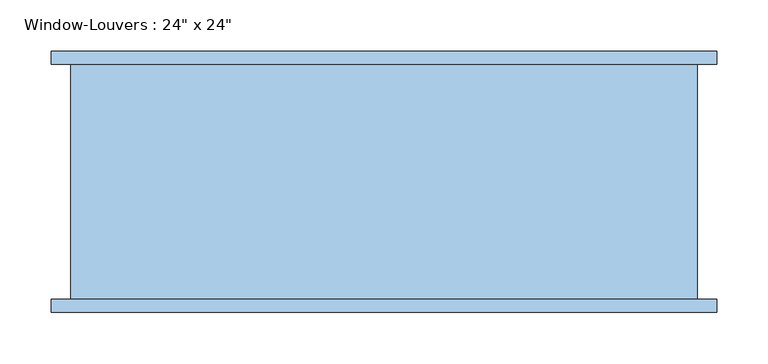
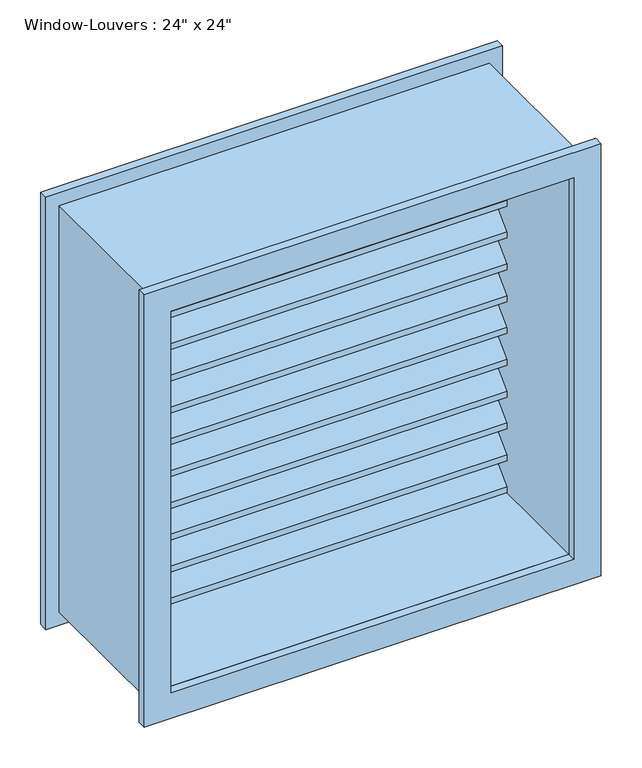
"""IFC4 building model written with IfcOpenShell, lengths in millimetres: window geometry."""

from ifc_helpers import new_model, si_unit, frame, origin, place, context, project, spatial, polyline, outline, extrude, source, transform, mapped, element, save


def window_f2d8fef0(model_context):
    return source(origin(), model_context, "Body", "SweptSolid", [
        extrude(outline(polyline([(107.95, 1419.1754778), (107.95, 1410.1952217), (69.85, 1448.2952217), (31.75, 1410.1952217), (31.75, 1419.1754778), (69.85, 1457.2754778), (107.95, 1419.1754778)])), frame((-285.75, 0.0, 0.0), z_axis=(1.0, 0.0, 0.0), x_axis=(0.0, 1.0, 0.0)), (0.0, 0.0, 1.0), 571.5),
        extrude(outline(polyline([(107.95, 1371.5009557), (107.95, 1362.5206995), (69.85, 1400.6206995), (31.75, 1362.5206995), (31.75, 1371.5009557), (69.85, 1409.6009557), (107.95, 1371.5009557)])), frame((-285.75, 0.0, 0.0), z_axis=(1.0, 0.0, 0.0), x_axis=(0.0, 1.0, 0.0)), (0.0, 0.0, 1.0), 571.5),
        extrude(outline(polyline([(107.95, 1323.8264335), (107.95, 1314.8461774), (69.85, 1352.9461774), (31.75, 1314.8461774), (31.75, 1323.8264335), (69.85, 1361.9264335), (107.95, 1323.8264335)])), frame((-285.75, 0.0, 0.0), z_axis=(1.0, 0.0, 0.0), x_axis=(0.0, 1.0, 0.0)), (0.0, 0.0, 1.0), 571.5),
        extrude(outline(polyline([(107.95, 1276.1519113), (107.95, 1267.1716552), (69.85, 1305.2716552), (31.75, 1267.1716552), (31.75, 1276.1519113), (69.85, 1314.2519113), (107.95, 1276.1519113)])), frame((-285.75, 0.0, 0.0), z_axis=(1.0, 0.0, 0.0), x_axis=(0.0, 1.0, 0.0)), (0.0, 0.0, 1.0), 571.5),
        extrude(outline(polyline([(107.95, 1228.4773891), (107.95, 1219.497133), (69.85, 1257.597133), (31.75, 1219.497133), (31.75, 1228.4773891), (69.85, 1266.5773891), (107.95, 1228.4773891)])), frame((-285.75, 0.0, 0.0), z_axis=(1.0, 0.0, 0.0), x_axis=(0.0, 1.0, 0.0)), (0.0, 0.0, 1.0), 571.5),
        extrude(outline(polyline([(107.95, 1180.802867), (107.95, 1171.8226109), (69.85, 1209.9226109), (31.75, 1171.8226109), (31.75, 1180.802867), (69.85, 1218.902867), (107.95, 1180.802867)])), frame((-285.75, 0.0, 0.0), z_axis=(1.0, 0.0, 0.0), x_axis=(0.0, 1.0, 0.0)), (0.0, 0.0, 1.0), 571.5),
        extrude(outline(polyline([(107.95, 1133.1283448), (107.95, 1124.1480887), (69.85, 1162.2480887), (31.75, 1124.1480887), (31.75, 1133.1283448), (69.85, 1171.2283448), (107.95, 1133.1283448)])), frame((-285.75, 0.0, 0.0), z_axis=(1.0, 0.0, 0.0), x_axis=(0.0, 1.0, 0.0)), (0.0, 0.0, 1.0), 571.5),
        extrude(outline(polyline([(107.95, 1085.4538226), (107.95, 1076.4735665), (69.85, 1114.5735665), (31.75, 1076.4735665), (31.75, 1085.4538226), (69.85, 1123.5538226), (107.95, 1085.4538226)])), frame((-285.75, 0.0, 0.0), z_axis=(1.0, 0.0, 0.0), x_axis=(0.0, 1.0, 0.0)), (0.0, 0.0, 1.0), 571.5),
        extrude(outline(polyline([(107.95, 1037.7793005), (107.95, 1028.7990443), (69.85, 1066.8990443), (31.75, 1028.7990443), (31.75, 1037.7793005), (69.85, 1075.8793005), (107.95, 1037.7793005)])), frame((-285.75, 0.0, 0.0), z_axis=(1.0, 0.0, 0.0), x_axis=(0.0, 1.0, 0.0)), (0.0, 0.0, 1.0), 571.5),
        extrude(outline(polyline([(107.95, 990.1047783), (107.95, 981.1245222), (69.85, 1019.2245222), (31.75, 981.1245222), (31.75, 990.1047783), (69.85, 1028.2047783), (107.95, 990.1047783)])), frame((-285.75, 0.0, 0.0), z_axis=(1.0, 0.0, 0.0), x_axis=(0.0, 1.0, 0.0)), (0.0, 0.0, 1.0), 571.5),
        extrude(outline(polyline([(107.95, 1466.85), (107.95, 1457.8697439), (69.85, 1495.9697439), (31.75, 1457.8697439), (31.75, 1466.85), (69.85, 1504.95), (107.95, 1466.85)])), frame((-285.75, 0.0, 0.0), z_axis=(1.0, 0.0, 0.0), x_axis=(0.0, 1.0, 0.0)), (0.0, 0.0, 1.0), 571.5),
        extrude(outline(polyline([(107.95, 942.4302561), (107.95, 933.45), (69.85, 971.55), (31.75, 933.45), (31.75, 942.4302561), (69.85, 980.5302561), (107.95, 942.4302561)])), frame((-285.75, 0.0, 0.0), z_axis=(1.0, 0.0, 0.0), x_axis=(0.0, 1.0, 0.0)), (0.0, 0.0, 1.0), 571.5),
        extrude(outline(polyline([(1524.0, 304.8), (1524.0, -304.8), (914.4, -304.8), (914.4, 304.8), (1524.0, 304.8)]), holes=[polyline([(1504.95, 285.75), (933.45, 285.75), (933.45, -285.75), (1504.95, -285.75), (1504.95, 285.75)])]), frame((0.0, -120.65, 0.0), z_axis=(0.0, 1.0, 0.0), x_axis=(0.0, 0.0, 1.0)), (0.0, 0.0, 1.0), 228.6),
        extrude(outline(polyline([(1543.05, 323.85), (1543.05, -323.85), (895.35, -323.85), (895.35, 323.85), (1543.05, 323.85)]), holes=[polyline([(1504.95, 285.75), (933.45, 285.75), (933.45, -285.75), (1504.95, -285.75), (1504.95, 285.75)])]), frame((0.0, -133.35, 0.0), z_axis=(0.0, 1.0, 0.0), x_axis=(0.0, 0.0, 1.0)), (0.0, 0.0, 1.0), 12.7),
        extrude(outline(polyline([(1543.05, -323.85), (895.35, -323.85), (895.35, 323.85), (1543.05, 323.85), (1543.05, -323.85)]), holes=[polyline([(1504.95, -285.75), (1504.95, 285.75), (933.45, 285.75), (933.45, -285.75), (1504.95, -285.75)])]), frame((0.0, 107.95, 0.0), z_axis=(0.0, 1.0, 0.0), x_axis=(0.0, 0.0, 1.0)), (0.0, 0.0, 1.0), 12.7),
    ])


if __name__ == "__main__":
    model = new_model("IFC4")
    model_context = context("Model", 3, world=origin())
    ifc_project = project(units=[si_unit("LENGTHUNIT", "METRE", prefix="MILLI")], contexts=[model_context])
    site = spatial("IfcSite", under=ifc_project)
    building = spatial("IfcBuilding", under=site)
    placement = place(None, origin())
    window_shape = window_f2d8fef0(model_context)
    element("IfcWindow", 1, ObjectType="Window-Louvers : 24\" x 24\"", at=placement, inside=building, context=model_context, shape_type="MappedRepresentation", body=[
        mapped(window_shape, transform((0.0, 0.0, 0.0), x_axis=(1.0, 0.0, 0.0), y_axis=(0.0, 1.0, 0.0), z_axis=(0.0, 0.0, 1.0))),
    ])
    save(model, "model.ifc")

# Revit data of these elements
# Type "Window-Louvers : 24\" x 24\""
#   Type Mark = "24"
#   Construction Type Id = "GSP4R"
#   Assembly Code = "B20"
#   Analytic Construction = "1/8 in Pilkington single glazing"
#   Visual Light Transmittance = 0.9
#   Thermal Resistance (R) = 1.53941 (h·ft²·°F)/BTU
#   Solar Heat Gain Coefficient = 0.78
#   Max Height = 1' - 11.74264"
#   Height = 2' - 0"
#   Heat Transfer Coefficient (U) = 0.6496 BTU/(h·ft²·°F)
#   Blade Width [instance default] = 1' - 10 1/2"
#   Blade Vertical Thickness = 0' - 0.35355"
#   Blade Thickness = 0' - 0 1/4"
#   Blade Spacing = 0' - 1 1/2"
#   Blade Height = 0' - 1.85355"
#   Blade Depth = 0' - 3"
#   Blade Angle = 45.00°
#   Default Sill Height = 3' - 0"
#   Trim Projection_Exterior = 0' - 0 1/2"
#   Trim Projection_Interior = 0' - 0 1/2"
#   Trim Width_Exterior = 0' - 1 1/2"
#   Trim Width_Interior = 0' - 1 1/2"
#   Width = 2' - 0"
#   Max Blade Count = 12
#   Define Thermal Properties by = 1
#   Blade Count = 12
#   Frame Material = Birch
#   Louver Material = Birch
#   Trim Exterior Material = Birch
#   Trim Interior Material = Birch
#   Wall Closure = (empty or 0)
# Element 1 (IfcWindow, "Window-Louvers : 24\" x 24\"")
#   Materials on its faces: "Birch"
# Materials
#   "Birch": class "Wood", colour RGB 224 178 126, transparency 0, Description = "Betula Alleghaniensis", Cost = 0
